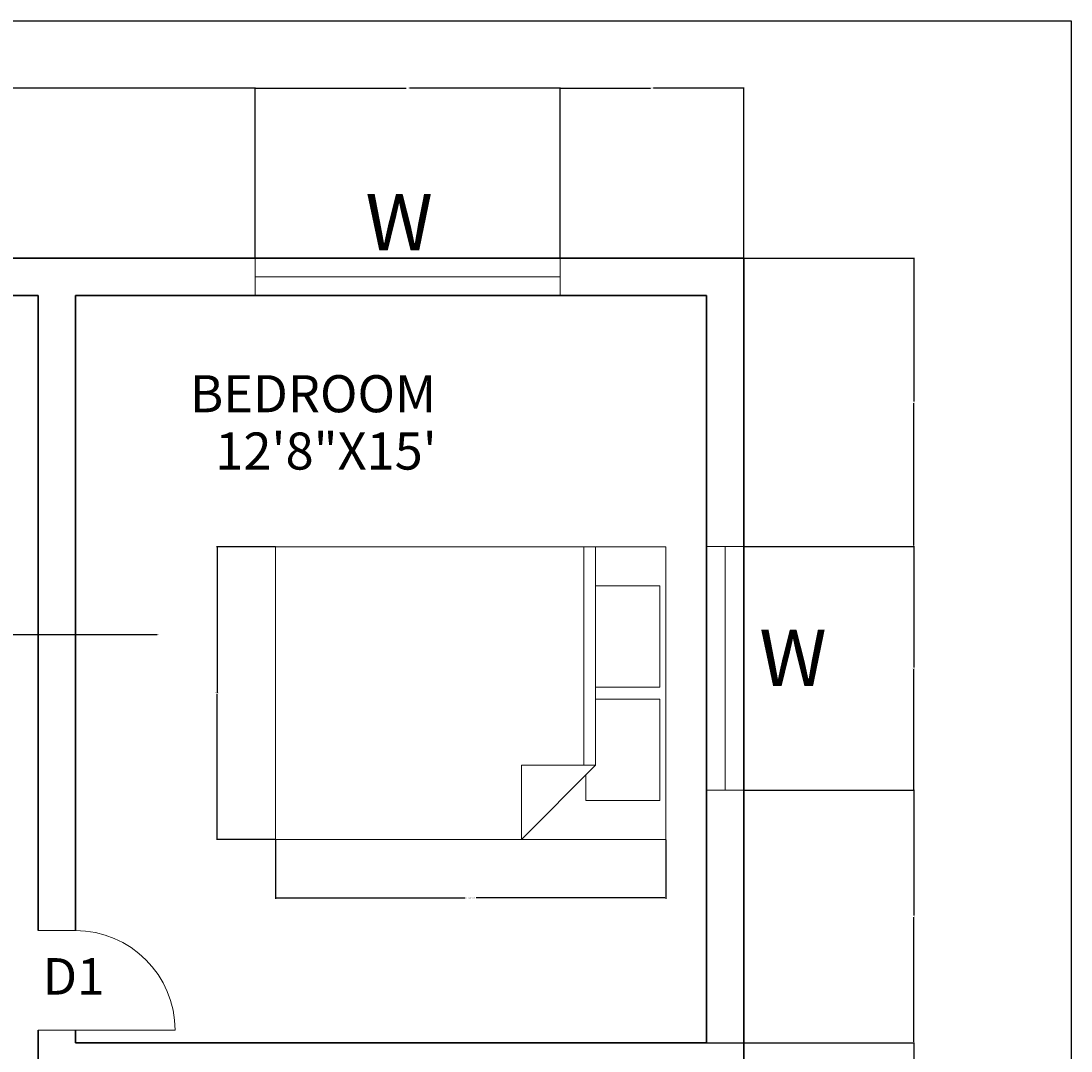
# Model space of a CAD drawing. Units: feet. Extents: x 1755 to 2628, y 1710 to 2329.
# Tile 4 of 4: x 2375 to 2628, y 2081 to 2329. Entities that reach past the tile are written whole.
import ezdxf

# ---------------------------------------------------------------- set-up
doc = ezdxf.new("R2010")
doc.units = ezdxf.units.FT
for name, color, linetype, lineweight in [('A-ANNO-DIMS', 2, 'Continuous', 18), ('A-ANNO-TEXT', 7, 'Continuous', 18), ('A-ANNO-TTLB', 7, 'Continuous', 25), ('A-AREA-IDEN', 7, 'Continuous', 18), ('A-DOOR', 3, 'Continuous', 18), ('A-FURN', 8, 'Continuous', 18), ('A-GLAZ', 4, 'Continuous', 18), ('A-WALL', 7, 'Continuous', 35)]:
    doc.layers.add(name, color=color, linetype=linetype, lineweight=lineweight)
doc.styles.get("Standard").update_dxf_attribs({"font": 'arial.ttf'})
doc.dimstyles.get("Standard").update_dxf_attribs({"dimtxt": 0.18, "dimasz": 0.18, "dimexe": 0.18, "dimexo": 0.0625, "dimgap": 0.09, "dimtad": 0, "dimtih": 1, "dimtoh": 1, "dimdec": 4, "dimzin": 0, "dimdsep": 46, "dimtxsty": 'Standard', "dimcen": 0.09, "dimadec": 0, "dimazin": 0, "dimtfac": 1, "dimtdec": 4, "dimtofl": 0, "dimtmove": 0, "dimatfit": 3, "dimfxl": 1, "dimtolj": 1, "dimtzin": 0, "dimarcsym": 0})

# ---------------------------------------------------------------- blocks, each defined once
blk = doc.blocks.new('Bed - Queen')
for p, q in [((0, -80.00003), (0, 0)), ((0, 0), (59.99999, 0)), ((59.99999, 0), (59.99999, -80.00003)), ((7.99999, -1.2), (28.79998, -1.2)), ((7.99999, -14.4), (7.99999, -1.2)), ((28.79998, -1.2), (28.79998, -14.4)), ((31.19999, -1.2), (51.99999, -1.2)), ((31.19999, -14.4), (31.19999, -1.2)), ((51.99999, -1.2), (51.99999, -16.4)), ((0, -14.4), (44.8, -14.4)), ((59.99999, -29.6), (44.8, -14.4)), ((44.8, -14.4), (44.8, -29.6)), ((44.8, -16.8), (0, -16.8)), ((51.99999, -16.4), (46.79936, -16.4)), ((44.8, -29.6), (59.99999, -29.6)), ((59.99999, -80.00003), (0, -80.00003))]:
    blk.add_line(p, q)
blk = doc.blocks.new('DOOR-SINGLE-SWING')
for p, q in [((0, 33), (0, 0)), ((24, 9), (24, 0))]:
    blk.add_line(p, q)
blk.add_arc((0, 9), 24, 0, 90)
blk = doc.blocks.new('*D10')
at = {"layer": 'A-ANNO-DIMS', "color": 0, "lineweight": -2, "transparency": 16777216}
for p, q in [((2436.11, 2131.72), (2436.11, 2117.51)), ((2530.08, 2131.72), (2530.08, 2117.51)), ((2436.29, 2117.69), (2481.79, 2117.69)), ((2529.9, 2117.69), (2484.4, 2117.69))]:
    blk.add_line(p, q, dxfattribs=at)
at = {"layer": 'A-ANNO-DIMS', "color": 0, "transparency": 16777216}
for points in [[(2436.29, 2117.72), (2436.29, 2117.66), (2436.11, 2117.69)], [(2529.9, 2117.72), (2529.9, 2117.66), (2530.08, 2117.69)]]:
    blk.add_solid(points, dxfattribs=at)
at = {"layer": 'Defpoints', "color": 0, "transparency": 16777216}
for p in [(2436.11, 2131.78), (2530.08, 2131.78), (2530.08, 2117.69)]:
    blk.add_point(p, dxfattribs=at)
at = {"layer": 'A-ANNO-DIMS', "color": 0, "transparency": 16777216, "insert": (2483.09, 2117.69), "char_height": 0.18, "attachment_point": 5}
blk.add_mtext('\\A1;QUEEN BED 94 TYP.', dxfattribs=at)
blk = doc.blocks.new('*D11')
at = {"layer": 'A-ANNO-DIMS', "color": 0, "lineweight": -2, "transparency": 16777216}
for p, q in [((2436.05, 2202.25), (2421.84, 2202.25)), ((2422.02, 2202.07), (2422.02, 2167.2)), ((2422.02, 2131.96), (2422.02, 2166.83)), ((2436.05, 2131.78), (2421.84, 2131.78))]:
    blk.add_line(p, q, dxfattribs=at)
at = {"layer": 'A-ANNO-DIMS', "color": 0, "transparency": 16777216}
for points in [[(2421.99, 2202.07), (2422.05, 2202.07), (2422.02, 2202.25)], [(2421.99, 2131.96), (2422.05, 2131.96), (2422.02, 2131.78)]]:
    blk.add_solid(points, dxfattribs=at)
at = {"layer": 'Defpoints', "color": 0, "transparency": 16777216}
for p in [(2436.11, 2202.25), (2422.02, 2131.78), (2436.11, 2131.78)]:
    blk.add_point(p, dxfattribs=at)
at = {"layer": 'A-ANNO-DIMS', "color": 0, "transparency": 16777216, "insert": (2422.02, 2167.02), "char_height": 0.18, "attachment_point": 5}
blk.add_mtext('\\A1;70 TYP.', dxfattribs=at)
blk = doc.blocks.new('*D28')
at = {"layer": 'A-ANNO-DIMS', "color": 0, "lineweight": -2, "transparency": 16777216}
for p, q in [((2296.06, 2271.88), (2296.06, 2312.95)), ((2296.24, 2312.77), (2363.18, 2312.77)), ((2431.02, 2312.77), (2364.09, 2312.77)), ((2431.2, 2271.88), (2431.2, 2312.95))]:
    blk.add_line(p, q, dxfattribs=at)
at = {"layer": 'A-ANNO-DIMS', "color": 0, "transparency": 16777216}
for points in [[(2296.24, 2312.8), (2296.24, 2312.74), (2296.06, 2312.77)], [(2431.02, 2312.8), (2431.02, 2312.74), (2431.2, 2312.77)]]:
    blk.add_solid(points, dxfattribs=at)
at = {"layer": 'Defpoints', "color": 0, "transparency": 16777216}
for p in [(2431.2, 2312.77), (2296.06, 2271.82), (2431.2, 2271.82)]:
    blk.add_point(p, dxfattribs=at)
at = {"layer": 'A-ANNO-DIMS', "color": 0, "transparency": 16777216, "insert": (2363.63, 2312.77), "char_height": 0.18, "attachment_point": 5}
blk.add_mtext('\\A1;135.14', dxfattribs=at)
blk = doc.blocks.new('*D29')
at = {"layer": 'A-ANNO-DIMS', "color": 0, "lineweight": -2, "transparency": 16777216}
for p, q in [((2431.2, 2271.88), (2431.2, 2312.95)), ((2431.38, 2312.77), (2467.54, 2312.77)), ((2504.48, 2312.77), (2468.33, 2312.77)), ((2504.66, 2271.88), (2504.66, 2312.95))]:
    blk.add_line(p, q, dxfattribs=at)
at = {"layer": 'A-ANNO-DIMS', "color": 0, "transparency": 16777216}
for points in [[(2431.38, 2312.8), (2431.38, 2312.74), (2431.2, 2312.77)], [(2504.48, 2312.8), (2504.48, 2312.74), (2504.66, 2312.77)]]:
    blk.add_solid(points, dxfattribs=at)
at = {"layer": 'Defpoints', "color": 0, "transparency": 16777216}
for p in [(2504.66, 2312.77), (2431.2, 2271.82), (2504.66, 2271.82)]:
    blk.add_point(p, dxfattribs=at)
at = {"layer": 'A-ANNO-DIMS', "color": 0, "transparency": 16777216, "insert": (2467.93, 2312.77), "char_height": 0.18, "attachment_point": 5}
blk.add_mtext('\\A1;73.46', dxfattribs=at)
blk = doc.blocks.new('*D30')
at = {"layer": 'A-ANNO-DIMS', "color": 0, "lineweight": -2, "transparency": 16777216}
for p, q in [((2504.66, 2271.88), (2504.66, 2312.95)), ((2504.84, 2312.77), (2526.38, 2312.77)), ((2548.71, 2312.77), (2527.17, 2312.77)), ((2548.89, 2271.88), (2548.89, 2312.95))]:
    blk.add_line(p, q, dxfattribs=at)
at = {"layer": 'A-ANNO-DIMS', "color": 0, "transparency": 16777216}
for points in [[(2504.84, 2312.8), (2504.84, 2312.74), (2504.66, 2312.77)], [(2548.71, 2312.8), (2548.71, 2312.74), (2548.89, 2312.77)]]:
    blk.add_solid(points, dxfattribs=at)
at = {"layer": 'Defpoints', "color": 0, "transparency": 16777216}
for p in [(2548.89, 2312.77), (2504.66, 2271.82), (2548.89, 2271.82)]:
    blk.add_point(p, dxfattribs=at)
at = {"layer": 'A-ANNO-DIMS', "color": 0, "transparency": 16777216, "insert": (2526.78, 2312.77), "char_height": 0.18, "attachment_point": 5}
blk.add_mtext('\\A1;44.23', dxfattribs=at)
blk = doc.blocks.new('*D31')
at = {"layer": 'A-ANNO-DIMS', "color": 0, "lineweight": -2, "transparency": 16777216}
for p, q in [((2548.95, 2271.82), (2590.02, 2271.82)), ((2589.84, 2271.64), (2589.84, 2237.28)), ((2589.84, 2202.55), (2589.84, 2236.91)), ((2548.95, 2202.37), (2590.02, 2202.37))]:
    blk.add_line(p, q, dxfattribs=at)
at = {"layer": 'A-ANNO-DIMS', "color": 0, "transparency": 16777216}
for points in [[(2589.81, 2271.64), (2589.87, 2271.64), (2589.84, 2271.82)], [(2589.81, 2202.55), (2589.87, 2202.55), (2589.84, 2202.37)]]:
    blk.add_solid(points, dxfattribs=at)
at = {"layer": 'Defpoints', "color": 0, "transparency": 16777216}
for p in [(2548.89, 2271.82), (2548.89, 2202.37), (2589.84, 2202.37)]:
    blk.add_point(p, dxfattribs=at)
at = {"layer": 'A-ANNO-DIMS', "color": 0, "transparency": 16777216, "insert": (2589.84, 2237.09), "char_height": 0.18, "attachment_point": 5}
blk.add_mtext('\\A1;69.44', dxfattribs=at)
blk = doc.blocks.new('*D32')
at = {"layer": 'A-ANNO-DIMS', "color": 0, "lineweight": -2, "transparency": 16777216}
for p, q in [((2548.95, 2202.37), (2590.02, 2202.37)), ((2589.84, 2202.19), (2589.84, 2173.2)), ((2589.84, 2143.84), (2589.84, 2172.83)), ((2548.95, 2143.66), (2590.02, 2143.66))]:
    blk.add_line(p, q, dxfattribs=at)
at = {"layer": 'A-ANNO-DIMS', "color": 0, "transparency": 16777216}
for points in [[(2589.81, 2202.19), (2589.87, 2202.19), (2589.84, 2202.37)], [(2589.81, 2143.84), (2589.87, 2143.84), (2589.84, 2143.66)]]:
    blk.add_solid(points, dxfattribs=at)
at = {"layer": 'Defpoints', "color": 0, "transparency": 16777216}
for p in [(2548.89, 2202.37), (2548.89, 2143.66), (2589.84, 2143.66)]:
    blk.add_point(p, dxfattribs=at)
at = {"layer": 'A-ANNO-DIMS', "color": 0, "transparency": 16777216, "insert": (2589.84, 2173.02), "char_height": 0.18, "attachment_point": 5}
blk.add_mtext('\\A1;58.71', dxfattribs=at)
blk = doc.blocks.new('*D33')
at = {"layer": 'A-ANNO-DIMS', "color": 0, "lineweight": -2, "transparency": 16777216}
for p, q in [((2548.95, 2143.66), (2590.02, 2143.66)), ((2589.84, 2143.48), (2589.84, 2113.42)), ((2589.84, 2083), (2589.84, 2113.06)), ((2539.95, 2082.82), (2590.02, 2082.82))]:
    blk.add_line(p, q, dxfattribs=at)
at = {"layer": 'A-ANNO-DIMS', "color": 0, "transparency": 16777216}
for points in [[(2589.81, 2143.48), (2589.87, 2143.48), (2589.84, 2143.66)], [(2589.81, 2083), (2589.87, 2083), (2589.84, 2082.82)]]:
    blk.add_solid(points, dxfattribs=at)
at = {"layer": 'Defpoints', "color": 0, "transparency": 16777216}
for p in [(2548.89, 2143.66), (2539.89, 2082.82), (2589.84, 2082.82)]:
    blk.add_point(p, dxfattribs=at)
at = {"layer": 'A-ANNO-DIMS', "color": 0, "transparency": 16777216, "insert": (2589.84, 2113.24), "char_height": 0.18, "attachment_point": 5}
blk.add_mtext('\\A1;60.84', dxfattribs=at)
blk = doc.blocks.new('*D34')
at = {"layer": 'A-ANNO-DIMS', "color": 0, "lineweight": -2, "transparency": 16777216}
for p, q in [((2539.95, 2082.82), (2590.02, 2082.82)), ((2589.84, 2082.64), (2589.84, 1986)), ((2589.84, 1889), (2589.84, 1985.63)), ((2539.95, 1888.82), (2590.02, 1888.82))]:
    blk.add_line(p, q, dxfattribs=at)
at = {"layer": 'A-ANNO-DIMS', "color": 0, "transparency": 16777216}
for points in [[(2589.81, 2082.64), (2589.87, 2082.64), (2589.84, 2082.82)], [(2589.81, 1889), (2589.87, 1889), (2589.84, 1888.82)]]:
    blk.add_solid(points, dxfattribs=at)
at = {"layer": 'Defpoints', "color": 0, "transparency": 16777216}
for p in [(2539.89, 2082.82), (2539.89, 1888.82), (2589.84, 1888.82)]:
    blk.add_point(p, dxfattribs=at)
at = {"layer": 'A-ANNO-DIMS', "color": 0, "transparency": 16777216, "insert": (2589.84, 1985.82), "char_height": 0.18, "attachment_point": 5}
blk.add_mtext('\\A1;194', dxfattribs=at)
blk = doc.blocks.new('*D55')
at = {"layer": 'A-ANNO-DIMS', "color": 0, "lineweight": -2, "transparency": 16777216}
for p, q in [((2270.14, 2181.08), (2270.32, 2181.08)), ((2270.23, 2180.99), (2270.23, 2181.17)), ((2406.31, 2181.08), (2355.46, 2181.08))]:
    blk.add_line(p, q, dxfattribs=at)
at = {"layer": 'A-ANNO-DIMS', "color": 0, "transparency": 16777216}
blk.add_solid([(2355.46, 2181.11), (2355.46, 2181.05), (2355.28, 2181.08)], dxfattribs=at)
at = {"layer": 'Defpoints', "color": 0, "transparency": 16777216}
for p in [(2270.23, 2181.08), (2355.28, 2181.08)]:
    blk.add_point(p, dxfattribs=at)
at = {"layer": 'A-ANNO-DIMS', "color": 0, "transparency": 16777216, "insert": (2406.79, 2181.08), "char_height": 0.18, "attachment_point": 5}
blk.add_mtext('\\A1;R85.05', dxfattribs=at)
blk = doc.blocks.new('*D56')
at = {"layer": 'A-ANNO-DIMS', "color": 0, "lineweight": -2, "transparency": 16777216}
for p, q in [((2279.23, 2181.08), (2279.41, 2181.08)), ((2279.32, 2180.99), (2279.32, 2181.17)), ((2407.6, 2181.08), (2359.67, 2181.08))]:
    blk.add_line(p, q, dxfattribs=at)
at = {"layer": 'A-ANNO-DIMS', "color": 0, "transparency": 16777216}
blk.add_solid([(2359.67, 2181.11), (2359.67, 2181.05), (2359.49, 2181.08)], dxfattribs=at)
at = {"layer": 'Defpoints', "color": 0, "transparency": 16777216}
for p in [(2279.32, 2181.08), (2359.49, 2181.08)]:
    blk.add_point(p, dxfattribs=at)
at = {"layer": 'A-ANNO-DIMS', "color": 0, "transparency": 16777216, "insert": (2408.08, 2181.08), "char_height": 0.18, "attachment_point": 5}
blk.add_mtext('\\A1;R80.17', dxfattribs=at)

msp = doc.modelspace()

# ---------------------------------------------------------------- linework, layer by layer
at = {"layer": 'A-ANNO-TTLB'}
msp.add_lwpolyline([(1754.8706, 2328.9307), (2627.7013, 2328.9307), (2627.7013, 1709.9251), (1754.8706, 1709.9251)], close=True, dxfattribs=at)
at = {"layer": 'A-GLAZ'}
for p, q in [((2431.1999, 2271.8157), (2431.1999, 2262.8157)), ((2504.6643, 2271.8157), (2504.6643, 2262.8157)), ((2431.1999, 2267.3157), (2504.6643, 2267.3157)), ((2539.8905, 2202.3716), (2548.8905, 2202.3716)), ((2544.3905, 2202.3716), (2544.3905, 2143.6597)), ((2539.8905, 2143.6597), (2548.8905, 2143.6597))]:
    msp.add_line(p, q, dxfattribs=at)
at = {"layer": 'A-WALL'}
for p, q in [((2096.8905, 2271.8157), (2548.8905, 2271.8157)), ((2387.8905, 2271.8157), (2548.8905, 2271.8157)), ((2548.8905, 2271.8157), (2548.8905, 1834.8157)), ((2096.8905, 2262.8157), (2378.8905, 2262.8157)), ((2378.8905, 2262.8157), (2378.8905, 2109.8157)), ((2387.8905, 2262.8157), (2387.8905, 2109.8157)), ((2387.8905, 2262.8157), (2539.8905, 2262.8157)), ((2539.8905, 2262.8157), (2539.8905, 2082.8157)), ((2378.8905, 2085.8157), (2378.8905, 2078.8157)), ((2387.8905, 2085.8157), (2387.8905, 2082.8157)), ((2539.8905, 2082.8157), (2387.8905, 2082.8157))]:
    msp.add_line(p, q, dxfattribs=at)

# ---------------------------------------------------------------- block references
at = {"layer": 'A-DOOR', "extrusion": (0, 0, -1), "zscale": -1, "rotation": 90.00000000000342}
msp.add_blockref('DOOR-SINGLE-SWING', (-2378.8909, 2085.8161), dxfattribs=at)
at = {"layer": 'A-FURN', "xscale": 1.174519185879722, "yscale": 1.174519185879722, "zscale": 1.174519185879722, "rotation": 270}
msp.add_blockref('Bed - Queen', (2530.0752, 2202.2524), dxfattribs=at)

# ---------------------------------------------------------------- texts
at = {"layer": 'A-ANNO-TEXT'}
for s, height, p in [('W', 13.589, (2457.7239, 2273.6817)), ('W', 13.589, (2552.5913, 2168.7353)), ('D1', 8.79691, (2380.0269, 2094.3874))]:
    msp.add_text(s, height=height, dxfattribs=at).set_placement(p)
at = {"layer": 'A-AREA-IDEN'}
for s, p in [('BEDROOM', (2415.4925, 2234.6795)), ('12\'8"X15\'', (2421.5907, 2220.8752))]:
    msp.add_text(s, height=8.93153, dxfattribs=at).set_placement(p)

# ---------------------------------------------------------------- dimensions: what is measured, and where the dimension line sits
at = {"layer": 'A-ANNO-DIMS'}
for base, p1, p2, picture, middle in [((2431.1999, 2312.7657), (2296.063, 2271.8157), (2431.1999, 2271.8157), '*D28', (2363.6315, 2312.7657)), ((2504.6643, 2312.7657), (2431.1999, 2271.8157), (2504.6643, 2271.8157), '*D29', (2467.9321, 2312.7657)), ((2548.8905, 2312.7657), (2504.6643, 2271.8157), (2548.8905, 2271.8157), '*D30', (2526.7774, 2312.7657))]:
    dim = msp.add_linear_dim(base=base, p1=p1, p2=p2, dimstyle='Standard', override={"dimdec": 2, "dimlfac": 1, "dimrnd": 0, "dimzin": 0, "dimdsep": 46, "dimlunit": 2}, dxfattribs=at)
    dim.commit()
    dim.dimension.update_dxf_attribs({"geometry": picture, "text_midpoint": middle})
for base, p1, p2, override, picture, middle in [((2589.8405, 2202.3716), (2548.8905, 2271.8157), (2548.8905, 2202.3716), {"dimdec": 2, "dimlfac": 1, "dimrnd": 0, "dimzin": 0, "dimdsep": 46, "dimlunit": 2}, '*D31', (2589.8405, 2237.0936)), ((2589.8405, 2143.6597), (2548.8905, 2202.3716), (2548.8905, 2143.6597), {"dimdec": 2, "dimlfac": 1, "dimrnd": 0, "dimzin": 0, "dimdsep": 46, "dimlunit": 2}, '*D32', (2589.8405, 2173.0156)), ((2589.8405, 2082.8157), (2548.8905, 2143.6597), (2539.8905, 2082.8157), {"dimdec": 2, "dimlfac": 1, "dimrnd": 0, "dimzin": 0, "dimdsep": 46, "dimlunit": 2}, '*D33', (2589.8405, 2113.2377)), ((2589.8405, 1888.8157), (2539.8905, 2082.8157), (2539.8905, 1888.8157), {"dimdec": 0, "dimlfac": 1, "dimrnd": 0, "dimzin": 0, "dimdsep": 46, "dimlunit": 2}, '*D34', (2589.8405, 1985.8157))]:
    dim = msp.add_linear_dim(base=base, p1=p1, p2=p2, angle=90, dimstyle='Standard', override=override, dxfattribs=at)
    dim.commit()
    dim.dimension.update_dxf_attribs({"geometry": picture, "text_midpoint": middle})
dim = msp.add_linear_dim(base=(2422.0194, 2131.7813), p1=(2436.1136, 2202.2524), p2=(2436.1136, 2131.7813), angle=270, text='<> TYP.', dimstyle='Standard', override={"dimdec": 0, "dimlfac": 1, "dimrnd": 0, "dimzin": 0, "dimdsep": 46, "dimlunit": 2}, dxfattribs=at)
dim.commit()
dim.dimension.update_dxf_attribs({"geometry": '*D11', "text_midpoint": (2422.0194, 2167.0168)})
for center, mpoint, picture, middle in [((2270.2339, 2181.0761), (2355.2825, 2181.076), '*D55', (2406.3116, 2181.0759)), ((2279.3192, 2181.0761), (2359.4929, 2181.076), '*D56', (2407.5972, 2181.076))]:
    dim = msp.add_radius_dim(center=center, mpoint=mpoint, dimstyle='Standard', override={"dimdec": 2, "dimlfac": 1, "dimrnd": 0, "dimzin": 0, "dimdsep": 46, "dimlunit": 2}, dxfattribs=at)
    dim.commit()
    dim.dimension.update_dxf_attribs({"geometry": picture, "text_midpoint": middle, "dimtype": 164})
dim = msp.add_linear_dim(base=(2530.0752, 2117.687), p1=(2436.1136, 2131.7813), p2=(2530.0752, 2131.7813), text='QUEEN BED <> TYP.', dimstyle='Standard', override={"dimdec": 0, "dimlfac": 1, "dimrnd": 0, "dimzin": 0, "dimdsep": 46, "dimlunit": 2}, dxfattribs=at)
dim.commit()
dim.dimension.update_dxf_attribs({"geometry": '*D10', "text_midpoint": (2483.0944, 2117.687)})

doc.saveas('drawing.dxf')
